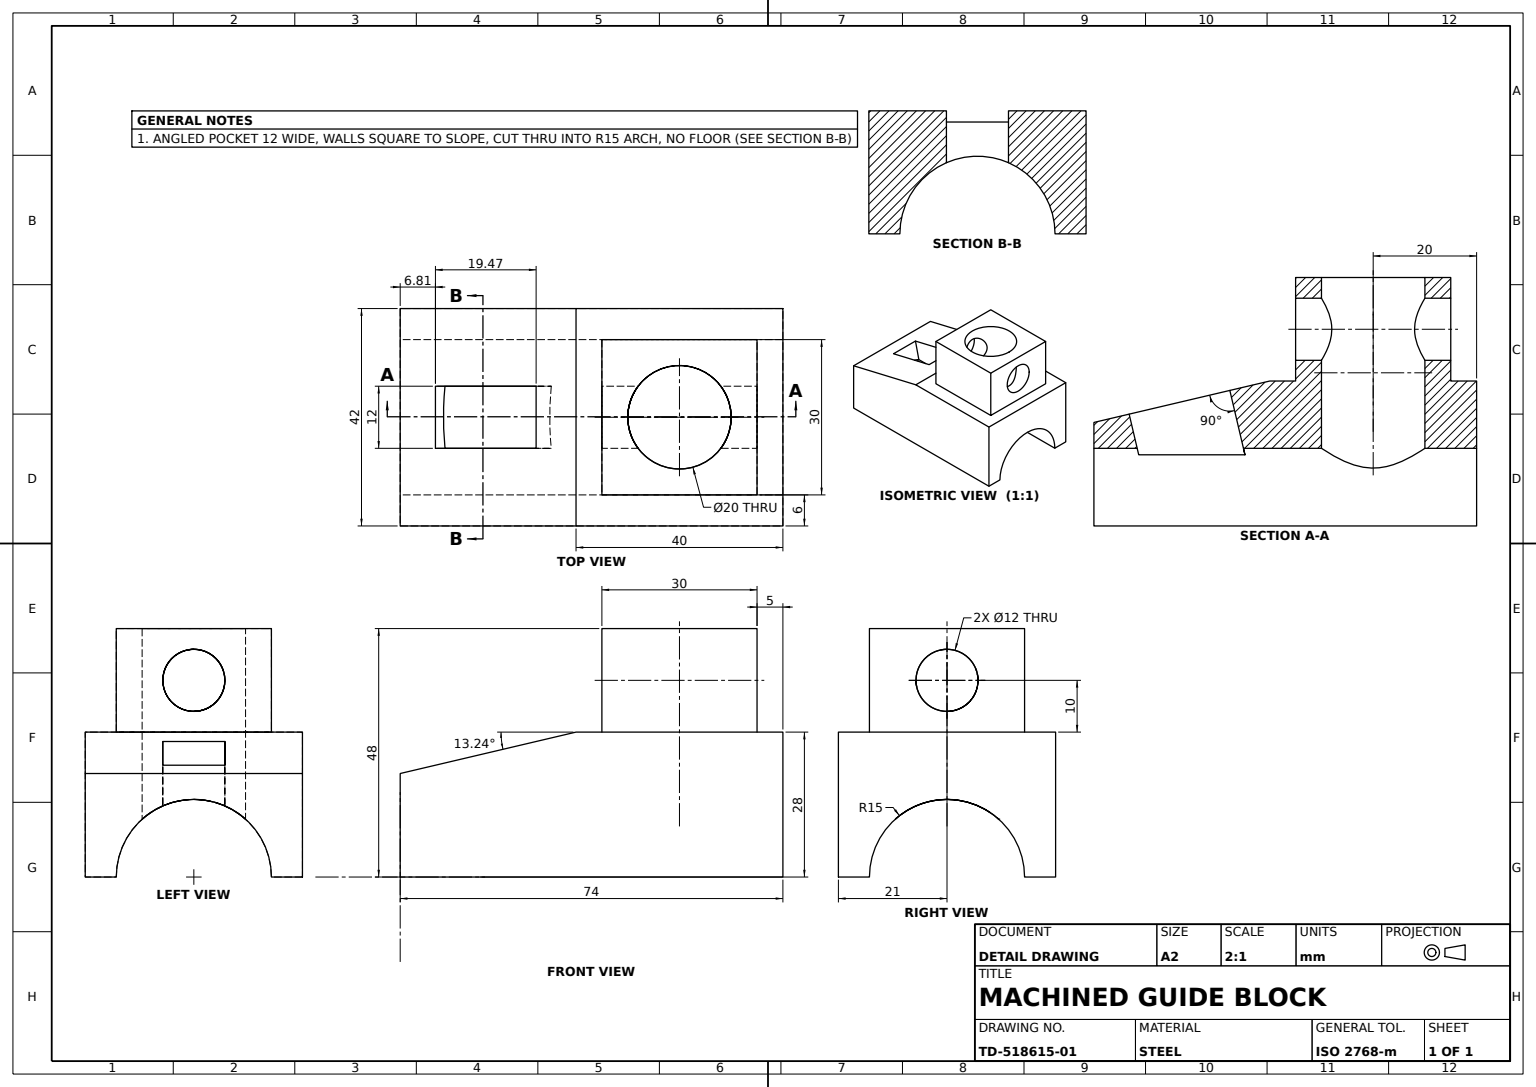
from build123d import *

# Parameters (mm, degrees)
BASE_BLOCK_DEPTH       = 42
TOP_BOSS_SKETCH_W      = 30
TOP_BOSS_SKETCH_H      = 30
TOP_BOSS_30X30_DEPTH   = 20
VERTICAL_BORE_SKETCH_R = 10
VERTICAL_BORE_DEPTH    = 98.693397935
CROSS_HOLE_SKETCH_R    = 6
CROSS_HOLE_DEPTH       = 75.759614766
ANGLED_POCKET_DEPTH    = 94.61448679
ARCH_CUTOUT_DEPTH      = 98.693397984
ARCH_CUTOUT_DEPTH_BACK = 98.693397984


with BuildPart() as part:
    # Base Block Profile Sketch → Base Block (new body)
    with BuildSketch(Plane.XY):
        Polygon((0, 0), (74, 0), (74, 28), (34, 28), (0, 20), align=None)
    extrude(amount=BASE_BLOCK_DEPTH)

    # Top Boss Sketch → Top Boss 30x30 (add)
    with BuildSketch(Plane(origin=(0, 28, 0), x_dir=(1, 0, 0), z_dir=(0, 1, 0))):
        with Locations((54, -21)):
            Rectangle(TOP_BOSS_SKETCH_W, TOP_BOSS_SKETCH_H)
    extrude(amount=TOP_BOSS_30X30_DEPTH)

    # Vertical Bore Sketch → Vertical Bore (cut, through all)
    with BuildSketch(Plane(origin=(0, 48, 0), x_dir=(1, 0, 0), z_dir=(0, 1, 0))):
        with Locations(Location((54, -21, 0), (0, 0, 180))):
            Circle(VERTICAL_BORE_SKETCH_R)
    extrude(amount=-VERTICAL_BORE_DEPTH, mode=Mode.SUBTRACT)

    # Cross Hole Sketch → Cross Hole (cut, through all)
    with BuildSketch(Plane.ZY.offset(-39)):
        with Locations((21, 38)):
            Circle(CROSS_HOLE_SKETCH_R)
    extrude(amount=-CROSS_HOLE_DEPTH, mode=Mode.SUBTRACT)

    # Angled Pocket Sketch → Angled Pocket (cut, through all)
    with BuildSketch(Plane(origin=(-4.459016393, 18.950819672, 0), x_dir=(0.973417168333576, 0.22903933372554744, 0), z_dir=(-0.22903933372554744, 0.973417168333576, 0))):
        Polygon((11.580786675, -21), (11.580786675, -15), (31.580786675, -15), (31.580786675, -27), (11.580786675, -27), align=None)
    extrude(amount=-ANGLED_POCKET_DEPTH, mode=Mode.SUBTRACT)

    # Arch Cutout Sketch → Arch Cutout (cut, two sides: drawn at the far end of the back side and taken through both)
    with BuildSketch(Plane.ZY.offset(-ARCH_CUTOUT_DEPTH_BACK)):
        with BuildLine():
            Line((36, -130.00000016), (36, 0))
            ThreePointArc((36, 0), (21, 15), (6, 0))
            Line((6, 0), (6, -130.00000016))
            Line((6, -130.00000016), (6, -390.00000048))
            Line((6, -390.00000048), (36, -390.00000048))
            Line((36, -390.00000048), (36, -130.00000016))
        make_face()
    extrude(amount=ARCH_CUTOUT_DEPTH + ARCH_CUTOUT_DEPTH_BACK, mode=Mode.SUBTRACT)


solid = part.part
